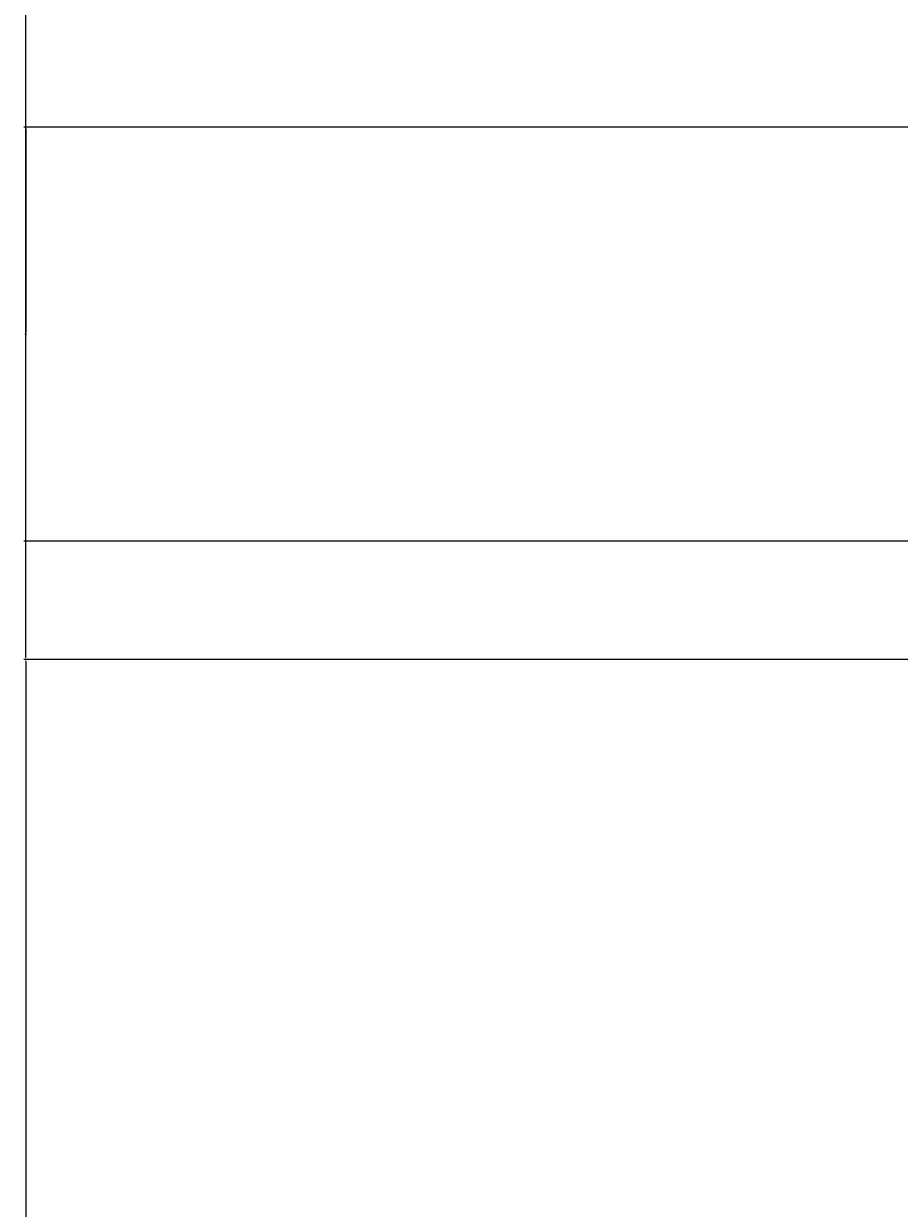
# Model space of a CAD drawing. Units: inches. Extents: x 5375 to 6084, y 16106 to 17259.
# Tile 19 of 32: x 5376 to 5464, y 16812 to 16932. Entities that reach past the tile are written whole.
import ezdxf

# ---------------------------------------------------------------- set-up
doc = ezdxf.new("R2010")
doc.units = ezdxf.units.IN
doc.layers.add('A-ANNO-DIMS', color=2, linetype='Continuous', lineweight=18)
doc.styles.get("Standard").update_dxf_attribs({"font": 'arial.ttf'})
doc.dimstyles.get("Standard").update_dxf_attribs({"dimtxt": 0.18, "dimasz": 0.18, "dimexe": 0.18, "dimexo": 0.0625, "dimgap": 0.09, "dimtad": 0, "dimtih": 1, "dimtoh": 1, "dimdec": 4, "dimzin": 0, "dimdsep": 46, "dimtxsty": 'Standard', "dimcen": 0.09, "dimadec": 0, "dimazin": 0, "dimtfac": 1, "dimtdec": 4, "dimtofl": 0, "dimtmove": 0, "dimatfit": 3, "dimfxl": 1, "dimtolj": 1, "dimtzin": 0, "dimarcsym": 0})

# ---------------------------------------------------------------- blocks, each defined once
blk = doc.blocks.new('*D36')
at = {"layer": 'A-ANNO-DIMS', "color": 0, "lineweight": -2, "transparency": 16777216}
for p, q in [((5544.56, 16867.58), (5375.56, 16867.58)), ((5375.74, 16867.4), (5375.74, 16783.76)), ((5375.74, 16699.76), (5375.74, 16783.4)), ((5544.56, 16699.58), (5375.56, 16699.58))]:
    blk.add_line(p, q, dxfattribs=at)
at = {"layer": 'A-ANNO-DIMS', "color": 0, "transparency": 16777216}
for points in [[(5375.71, 16867.4), (5375.77, 16867.4), (5375.74, 16867.58)], [(5375.71, 16699.76), (5375.77, 16699.76), (5375.74, 16699.58)]]:
    blk.add_solid(points, dxfattribs=at)
at = {"layer": 'Defpoints', "color": 0, "transparency": 16777216}
for p in [(5375.74, 16867.58), (5544.62, 16867.58), (5544.62, 16699.58)]:
    blk.add_point(p, dxfattribs=at)
at = {"layer": 'A-ANNO-DIMS', "color": 0, "transparency": 16777216, "insert": (5375.74, 16783.58), "char_height": 0.18, "attachment_point": 5}
blk.add_mtext('\\A1;168', dxfattribs=at)
blk = doc.blocks.new('*D37')
at = {"layer": 'A-ANNO-DIMS', "color": 0, "lineweight": -2, "transparency": 16777216}
for p, q in [((5520.56, 17206.58), (5375.56, 17206.58)), ((5375.74, 17206.4), (5375.74, 17037.26)), ((5375.74, 16867.76), (5375.74, 17036.9)), ((5520.56, 16867.58), (5375.56, 16867.58))]:
    blk.add_line(p, q, dxfattribs=at)
at = {"layer": 'A-ANNO-DIMS', "color": 0, "transparency": 16777216}
for points in [[(5375.71, 17206.4), (5375.77, 17206.4), (5375.74, 17206.58)], [(5375.71, 16867.76), (5375.77, 16867.76), (5375.74, 16867.58)]]:
    blk.add_solid(points, dxfattribs=at)
at = {"layer": 'Defpoints', "color": 0, "transparency": 16777216}
for p in [(5375.74, 17206.58), (5520.62, 17206.58), (5520.62, 16867.58)]:
    blk.add_point(p, dxfattribs=at)
at = {"layer": 'A-ANNO-DIMS', "color": 0, "transparency": 16777216, "insert": (5375.74, 17037.08), "char_height": 0.18, "attachment_point": 5}
blk.add_mtext('\\A1;339', dxfattribs=at)
blk = doc.blocks.new('*D42')
at = {"layer": 'A-ANNO-DIMS', "color": 0, "lineweight": -2, "transparency": 16777216}
for p, q in [((5826.06, 16921.58), (5375.56, 16921.58)), ((5375.74, 16921.4), (5375.74, 16900.76)), ((5375.74, 16879.76), (5375.74, 16900.4)), ((5826.06, 16879.58), (5375.56, 16879.58))]:
    blk.add_line(p, q, dxfattribs=at)
at = {"layer": 'A-ANNO-DIMS', "color": 0, "transparency": 16777216}
for points in [[(5375.71, 16921.4), (5375.77, 16921.4), (5375.74, 16921.58)], [(5375.71, 16879.76), (5375.77, 16879.76), (5375.74, 16879.58)]]:
    blk.add_solid(points, dxfattribs=at)
at = {"layer": 'Defpoints', "color": 0, "transparency": 16777216}
for p in [(5826.12, 16921.58), (5375.74, 16879.58), (5826.12, 16879.58)]:
    blk.add_point(p, dxfattribs=at)
at = {"layer": 'A-ANNO-DIMS', "color": 0, "transparency": 16777216, "insert": (5375.74, 16900.58), "char_height": 0.18, "attachment_point": 5}
blk.add_mtext('\\A1;42', dxfattribs=at)

msp = doc.modelspace()

# ---------------------------------------------------------------- dimensions: what is measured, and where the dimension line sits
at = {"layer": 'A-ANNO-DIMS'}
for base, p1, p2, picture, middle in [((5375.7423, 17206.5793), (5520.6199, 16867.5793), (5520.6199, 17206.5793), '*D37', (5375.7423, 17037.0793)), ((5375.7423, 16879.5793), (5826.1199, 16921.5793), (5826.1199, 16879.5793), '*D42', (5375.7423, 16900.5793)), ((5375.7423, 16867.5793), (5544.6199, 16699.5793), (5544.6199, 16867.5793), '*D36', (5375.7423, 16783.5793))]:
    dim = msp.add_linear_dim(base=base, p1=p1, p2=p2, angle=90, dimstyle='Standard', override={"dimdec": 0, "dimlfac": 1, "dimrnd": 0, "dimzin": 0, "dimdsep": 46, "dimlunit": 2}, dxfattribs=at)
    dim.commit()
    dim.dimension.update_dxf_attribs({"geometry": picture, "text_midpoint": middle})

doc.saveas('drawing.dxf')
